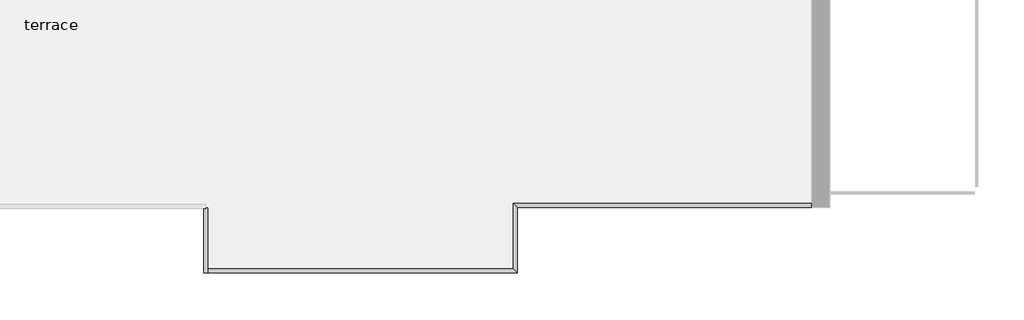
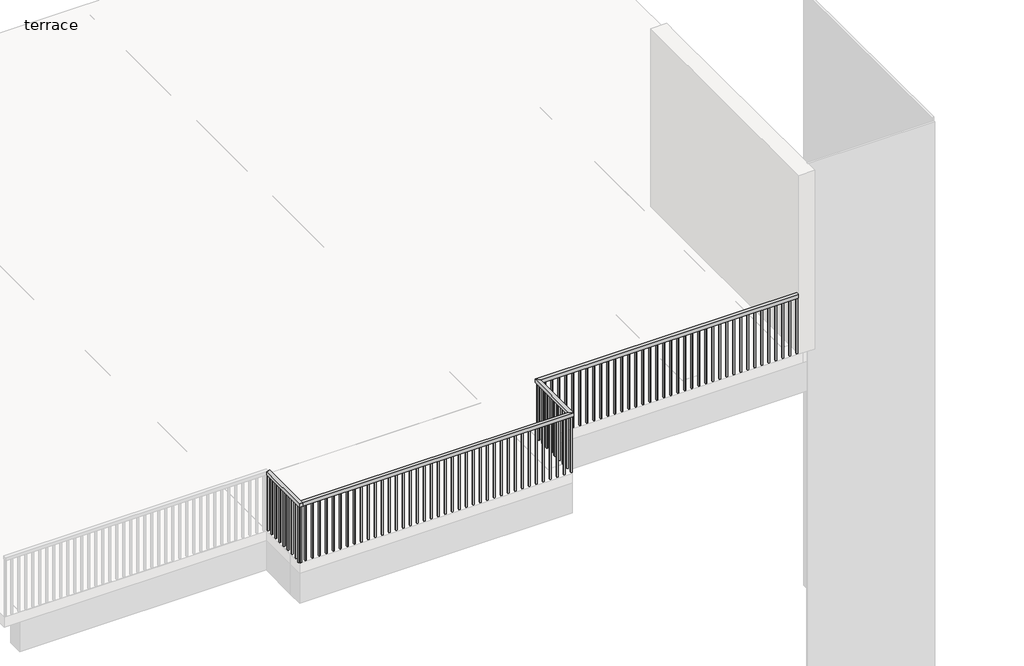
# One storey, part 3 of 6: 2 railings.
"""IFC4 building model written with IfcOpenShell, lengths in millimetres."""

from ifc_helpers import new_model, si_unit, frame, origin, place, context, project, spatial, polyline, outline, extrude, faceted_brep, element, save

model = new_model("IFC4")

# Units and contexts
model_context = context("Model", 3, world=origin())
ifc_project = project(units=[si_unit("LENGTHUNIT", "METRE", prefix="MILLI")], contexts=[model_context])

# Site, building, storey
site = spatial("IfcSite", under=ifc_project)
building = spatial("IfcBuilding", under=site)
storey = spatial("IfcBuildingStorey", under=building, Name="terrace", Elevation=7010.4)

# Railings
placement = place(None, origin())
element("IfcRailing", 1, ObjectType="Handrail - Rectangular", at=placement, inside=storey, context=model_context, shape_type="SweptSolid", body=[
    extrude(outline(polyline([(-12496.9493763, -4611.6564015), (-12446.1493763, -4611.6564015), (-12446.1493763, -5443.5064015), (-12496.9493763, -5443.5064015), (-12496.9493763, -4611.6564015)])), frame((0.0, 0.0, 7874.0), z_axis=(0.0, 0.0, 1.0), x_axis=(1.0, 0.0, 0.0)), (0.0, 0.0, 1.0), 50.8),
    extrude(outline(polyline([(-12481.0743763, -5414.9314015), (-12462.0243763, -5414.9314015), (-12462.0243763, -5433.9814015), (-12481.0743763, -5433.9814015), (-12481.0743763, -5414.9314015)])), frame((0.0, 0.0, 7010.4), z_axis=(0.0, 0.0, 1.0), x_axis=(1.0, 0.0, 0.0)), (0.0, 0.0, 1.0), 863.6),
    extrude(outline(polyline([(-12481.0743763, -5313.3314015), (-12462.0243763, -5313.3314015), (-12462.0243763, -5332.3814015), (-12481.0743763, -5332.3814015), (-12481.0743763, -5313.3314015)])), frame((0.0, 0.0, 7010.4), z_axis=(0.0, 0.0, 1.0), x_axis=(1.0, 0.0, 0.0)), (0.0, 0.0, 1.0), 863.6),
    extrude(outline(polyline([(-12481.0743763, -5211.7314015), (-12462.0243763, -5211.7314015), (-12462.0243763, -5230.7814015), (-12481.0743763, -5230.7814015), (-12481.0743763, -5211.7314015)])), frame((0.0, 0.0, 7010.4), z_axis=(0.0, 0.0, 1.0), x_axis=(1.0, 0.0, 0.0)), (0.0, 0.0, 1.0), 863.6),
    extrude(outline(polyline([(-12481.0743763, -5110.1314015), (-12462.0243763, -5110.1314015), (-12462.0243763, -5129.1814015), (-12481.0743763, -5129.1814015), (-12481.0743763, -5110.1314015)])), frame((0.0, 0.0, 7010.4), z_axis=(0.0, 0.0, 1.0), x_axis=(1.0, 0.0, 0.0)), (0.0, 0.0, 1.0), 863.6),
    extrude(outline(polyline([(-12481.0743763, -5008.5314015), (-12462.0243763, -5008.5314015), (-12462.0243763, -5027.5814015), (-12481.0743763, -5027.5814015), (-12481.0743763, -5008.5314015)])), frame((0.0, 0.0, 7010.4), z_axis=(0.0, 0.0, 1.0), x_axis=(1.0, 0.0, 0.0)), (0.0, 0.0, 1.0), 863.6),
    extrude(outline(polyline([(-12481.0743763, -4906.9314015), (-12462.0243763, -4906.9314015), (-12462.0243763, -4925.9814015), (-12481.0743763, -4925.9814015), (-12481.0743763, -4906.9314015)])), frame((0.0, 0.0, 7010.4), z_axis=(0.0, 0.0, 1.0), x_axis=(1.0, 0.0, 0.0)), (0.0, 0.0, 1.0), 863.6),
    extrude(outline(polyline([(-12481.0743763, -4805.3314015), (-12462.0243763, -4805.3314015), (-12462.0243763, -4824.3814015), (-12481.0743763, -4824.3814015), (-12481.0743763, -4805.3314015)])), frame((0.0, 0.0, 7010.4), z_axis=(0.0, 0.0, 1.0), x_axis=(1.0, 0.0, 0.0)), (0.0, 0.0, 1.0), 863.6),
    extrude(outline(polyline([(-12481.0743763, -4703.7314015), (-12462.0243763, -4703.7314015), (-12462.0243763, -4722.7814015), (-12481.0743763, -4722.7814015), (-12481.0743763, -4703.7314015)])), frame((0.0, 0.0, 7010.4), z_axis=(0.0, 0.0, 1.0), x_axis=(1.0, 0.0, 0.0)), (0.0, 0.0, 1.0), 863.6),
    extrude(outline(polyline([(-12481.0743763, -5424.4564015), (-12462.0243763, -5424.4564015), (-12462.0243763, -5443.5064015), (-12481.0743763, -5443.5064015), (-12481.0743763, -5424.4564015)])), frame((0.0, 0.0, 7010.4), z_axis=(0.0, 0.0, 1.0), x_axis=(1.0, 0.0, 0.0)), (0.0, 0.0, 1.0), 863.6),
    extrude(outline(polyline([(-12481.0743763, -4611.6564015), (-12462.0243763, -4611.6564015), (-12462.0243763, -4630.7064015), (-12481.0743763, -4630.7064015), (-12481.0743763, -4611.6564015)])), frame((0.0, 0.0, 7010.4), z_axis=(0.0, 0.0, 1.0), x_axis=(1.0, 0.0, 0.0)), (0.0, 0.0, 1.0), 863.6),
])
element("IfcRailing", 2, ObjectType="Handrail - Rectangular", at=placement, inside=storey, context=model_context, shape_type="SolidModel", body=[
    faceted_brep([(-12494.5077606, -5392.7064015, 7924.8), (-12494.5077606, -5392.7064015, 7874.0), (-12494.5077606, -5443.5064015, 7874.0), (-12494.5077606, -5443.5064015, 7924.8), (-8557.5077606, -5392.7064015, 7924.8), (-8557.5077606, -5392.7064015, 7874.0), (-8506.7077606, -5443.5064015, 7874.0), (-8506.7077606, -5443.5064015, 7924.8), (-8557.5077606, -4554.5064015, 7924.8), (-8557.5077606, -4554.5064015, 7874.0), (-8506.7077606, -4605.3064015, 7874.0), (-8506.7077606, -4605.3064015, 7924.8), (-4645.9077606, -4554.5064015, 7924.8), (-4645.9077606, -4605.3064015, 7924.8), (-4645.9077606, -4605.3064015, 7874.0), (-4645.9077606, -4554.5064015, 7874.0)], [[[0, 1, 2, 3]], [[1, 0, 4, 5]], [[2, 1, 5, 6]], [[3, 2, 6, 7]], [[0, 3, 7, 4]], [[5, 4, 8, 9]], [[6, 5, 9, 10]], [[7, 6, 10, 11]], [[4, 7, 11, 8]], [[12, 13, 14, 15]], [[9, 8, 12, 15]], [[10, 9, 15, 14]], [[11, 10, 14, 13]], [[8, 11, 13, 12]]]),
    extrude(outline(polyline([(-4680.8327606, -4589.4314015), (-4680.8327606, -4570.3814015), (-4661.7827606, -4570.3814015), (-4661.7827606, -4589.4314015), (-4680.8327606, -4589.4314015)])), frame((0.0, 0.0, 7010.4), z_axis=(0.0, 0.0, 1.0), x_axis=(1.0, 0.0, 0.0)), (0.0, 0.0, 1.0), 863.6),
    extrude(outline(polyline([(-4782.4327606, -4589.4314015), (-4782.4327606, -4570.3814015), (-4763.3827606, -4570.3814015), (-4763.3827606, -4589.4314015), (-4782.4327606, -4589.4314015)])), frame((0.0, 0.0, 7010.4), z_axis=(0.0, 0.0, 1.0), x_axis=(1.0, 0.0, 0.0)), (0.0, 0.0, 1.0), 863.6),
    extrude(outline(polyline([(-4884.0327606, -4589.4314015), (-4884.0327606, -4570.3814015), (-4864.9827606, -4570.3814015), (-4864.9827606, -4589.4314015), (-4884.0327606, -4589.4314015)])), frame((0.0, 0.0, 7010.4), z_axis=(0.0, 0.0, 1.0), x_axis=(1.0, 0.0, 0.0)), (0.0, 0.0, 1.0), 863.6),
    extrude(outline(polyline([(-4985.6327606, -4589.4314015), (-4985.6327606, -4570.3814015), (-4966.5827606, -4570.3814015), (-4966.5827606, -4589.4314015), (-4985.6327606, -4589.4314015)])), frame((0.0, 0.0, 7010.4), z_axis=(0.0, 0.0, 1.0), x_axis=(1.0, 0.0, 0.0)), (0.0, 0.0, 1.0), 863.6),
    extrude(outline(polyline([(-5087.2327606, -4589.4314015), (-5087.2327606, -4570.3814015), (-5068.1827606, -4570.3814015), (-5068.1827606, -4589.4314015), (-5087.2327606, -4589.4314015)])), frame((0.0, 0.0, 7010.4), z_axis=(0.0, 0.0, 1.0), x_axis=(1.0, 0.0, 0.0)), (0.0, 0.0, 1.0), 863.6),
    extrude(outline(polyline([(-5188.8327606, -4589.4314015), (-5188.8327606, -4570.3814015), (-5169.7827606, -4570.3814015), (-5169.7827606, -4589.4314015), (-5188.8327606, -4589.4314015)])), frame((0.0, 0.0, 7010.4), z_axis=(0.0, 0.0, 1.0), x_axis=(1.0, 0.0, 0.0)), (0.0, 0.0, 1.0), 863.6),
    extrude(outline(polyline([(-5290.4327606, -4589.4314015), (-5290.4327606, -4570.3814015), (-5271.3827606, -4570.3814015), (-5271.3827606, -4589.4314015), (-5290.4327606, -4589.4314015)])), frame((0.0, 0.0, 7010.4), z_axis=(0.0, 0.0, 1.0), x_axis=(1.0, 0.0, 0.0)), (0.0, 0.0, 1.0), 863.6),
    extrude(outline(polyline([(-5392.0327606, -4589.4314015), (-5392.0327606, -4570.3814015), (-5372.9827606, -4570.3814015), (-5372.9827606, -4589.4314015), (-5392.0327606, -4589.4314015)])), frame((0.0, 0.0, 7010.4), z_axis=(0.0, 0.0, 1.0), x_axis=(1.0, 0.0, 0.0)), (0.0, 0.0, 1.0), 863.6),
    extrude(outline(polyline([(-5493.6327606, -4589.4314015), (-5493.6327606, -4570.3814015), (-5474.5827606, -4570.3814015), (-5474.5827606, -4589.4314015), (-5493.6327606, -4589.4314015)])), frame((0.0, 0.0, 7010.4), z_axis=(0.0, 0.0, 1.0), x_axis=(1.0, 0.0, 0.0)), (0.0, 0.0, 1.0), 863.6),
    extrude(outline(polyline([(-5595.2327606, -4589.4314015), (-5595.2327606, -4570.3814015), (-5576.1827606, -4570.3814015), (-5576.1827606, -4589.4314015), (-5595.2327606, -4589.4314015)])), frame((0.0, 0.0, 7010.4), z_axis=(0.0, 0.0, 1.0), x_axis=(1.0, 0.0, 0.0)), (0.0, 0.0, 1.0), 863.6),
    extrude(outline(polyline([(-5696.8327606, -4589.4314015), (-5696.8327606, -4570.3814015), (-5677.7827606, -4570.3814015), (-5677.7827606, -4589.4314015), (-5696.8327606, -4589.4314015)])), frame((0.0, 0.0, 7010.4), z_axis=(0.0, 0.0, 1.0), x_axis=(1.0, 0.0, 0.0)), (0.0, 0.0, 1.0), 863.6),
    extrude(outline(polyline([(-5798.4327606, -4589.4314015), (-5798.4327606, -4570.3814015), (-5779.3827606, -4570.3814015), (-5779.3827606, -4589.4314015), (-5798.4327606, -4589.4314015)])), frame((0.0, 0.0, 7010.4), z_axis=(0.0, 0.0, 1.0), x_axis=(1.0, 0.0, 0.0)), (0.0, 0.0, 1.0), 863.6),
    extrude(outline(polyline([(-5900.0327606, -4589.4314015), (-5900.0327606, -4570.3814015), (-5880.9827606, -4570.3814015), (-5880.9827606, -4589.4314015), (-5900.0327606, -4589.4314015)])), frame((0.0, 0.0, 7010.4), z_axis=(0.0, 0.0, 1.0), x_axis=(1.0, 0.0, 0.0)), (0.0, 0.0, 1.0), 863.6),
    extrude(outline(polyline([(-6001.6327606, -4589.4314015), (-6001.6327606, -4570.3814015), (-5982.5827606, -4570.3814015), (-5982.5827606, -4589.4314015), (-6001.6327606, -4589.4314015)])), frame((0.0, 0.0, 7010.4), z_axis=(0.0, 0.0, 1.0), x_axis=(1.0, 0.0, 0.0)), (0.0, 0.0, 1.0), 863.6),
    extrude(outline(polyline([(-6103.2327606, -4589.4314015), (-6103.2327606, -4570.3814015), (-6084.1827606, -4570.3814015), (-6084.1827606, -4589.4314015), (-6103.2327606, -4589.4314015)])), frame((0.0, 0.0, 7010.4), z_axis=(0.0, 0.0, 1.0), x_axis=(1.0, 0.0, 0.0)), (0.0, 0.0, 1.0), 863.6),
    extrude(outline(polyline([(-6204.8327606, -4589.4314015), (-6204.8327606, -4570.3814015), (-6185.7827606, -4570.3814015), (-6185.7827606, -4589.4314015), (-6204.8327606, -4589.4314015)])), frame((0.0, 0.0, 7010.4), z_axis=(0.0, 0.0, 1.0), x_axis=(1.0, 0.0, 0.0)), (0.0, 0.0, 1.0), 863.6),
    extrude(outline(polyline([(-6306.4327606, -4589.4314015), (-6306.4327606, -4570.3814015), (-6287.3827606, -4570.3814015), (-6287.3827606, -4589.4314015), (-6306.4327606, -4589.4314015)])), frame((0.0, 0.0, 7010.4), z_axis=(0.0, 0.0, 1.0), x_axis=(1.0, 0.0, 0.0)), (0.0, 0.0, 1.0), 863.6),
    extrude(outline(polyline([(-6408.0327606, -4589.4314015), (-6408.0327606, -4570.3814015), (-6388.9827606, -4570.3814015), (-6388.9827606, -4589.4314015), (-6408.0327606, -4589.4314015)])), frame((0.0, 0.0, 7010.4), z_axis=(0.0, 0.0, 1.0), x_axis=(1.0, 0.0, 0.0)), (0.0, 0.0, 1.0), 863.6),
    extrude(outline(polyline([(-6509.6327606, -4589.4314015), (-6509.6327606, -4570.3814015), (-6490.5827606, -4570.3814015), (-6490.5827606, -4589.4314015), (-6509.6327606, -4589.4314015)])), frame((0.0, 0.0, 7010.4), z_axis=(0.0, 0.0, 1.0), x_axis=(1.0, 0.0, 0.0)), (0.0, 0.0, 1.0), 863.6),
    extrude(outline(polyline([(-6611.2327606, -4589.4314015), (-6611.2327606, -4570.3814015), (-6592.1827606, -4570.3814015), (-6592.1827606, -4589.4314015), (-6611.2327606, -4589.4314015)])), frame((0.0, 0.0, 7010.4), z_axis=(0.0, 0.0, 1.0), x_axis=(1.0, 0.0, 0.0)), (0.0, 0.0, 1.0), 863.6),
    extrude(outline(polyline([(-6712.8327606, -4589.4314015), (-6712.8327606, -4570.3814015), (-6693.7827606, -4570.3814015), (-6693.7827606, -4589.4314015), (-6712.8327606, -4589.4314015)])), frame((0.0, 0.0, 7010.4), z_axis=(0.0, 0.0, 1.0), x_axis=(1.0, 0.0, 0.0)), (0.0, 0.0, 1.0), 863.6),
    extrude(outline(polyline([(-6814.4327606, -4589.4314015), (-6814.4327606, -4570.3814015), (-6795.3827606, -4570.3814015), (-6795.3827606, -4589.4314015), (-6814.4327606, -4589.4314015)])), frame((0.0, 0.0, 7010.4), z_axis=(0.0, 0.0, 1.0), x_axis=(1.0, 0.0, 0.0)), (0.0, 0.0, 1.0), 863.6),
    extrude(outline(polyline([(-6916.0327606, -4589.4314015), (-6916.0327606, -4570.3814015), (-6896.9827606, -4570.3814015), (-6896.9827606, -4589.4314015), (-6916.0327606, -4589.4314015)])), frame((0.0, 0.0, 7010.4), z_axis=(0.0, 0.0, 1.0), x_axis=(1.0, 0.0, 0.0)), (0.0, 0.0, 1.0), 863.6),
    extrude(outline(polyline([(-7017.6327606, -4589.4314015), (-7017.6327606, -4570.3814015), (-6998.5827606, -4570.3814015), (-6998.5827606, -4589.4314015), (-7017.6327606, -4589.4314015)])), frame((0.0, 0.0, 7010.4), z_axis=(0.0, 0.0, 1.0), x_axis=(1.0, 0.0, 0.0)), (0.0, 0.0, 1.0), 863.6),
    extrude(outline(polyline([(-7119.2327606, -4589.4314015), (-7119.2327606, -4570.3814015), (-7100.1827606, -4570.3814015), (-7100.1827606, -4589.4314015), (-7119.2327606, -4589.4314015)])), frame((0.0, 0.0, 7010.4), z_axis=(0.0, 0.0, 1.0), x_axis=(1.0, 0.0, 0.0)), (0.0, 0.0, 1.0), 863.6),
    extrude(outline(polyline([(-7220.8327606, -4589.4314015), (-7220.8327606, -4570.3814015), (-7201.7827606, -4570.3814015), (-7201.7827606, -4589.4314015), (-7220.8327606, -4589.4314015)])), frame((0.0, 0.0, 7010.4), z_axis=(0.0, 0.0, 1.0), x_axis=(1.0, 0.0, 0.0)), (0.0, 0.0, 1.0), 863.6),
    extrude(outline(polyline([(-7322.4327606, -4589.4314015), (-7322.4327606, -4570.3814015), (-7303.3827606, -4570.3814015), (-7303.3827606, -4589.4314015), (-7322.4327606, -4589.4314015)])), frame((0.0, 0.0, 7010.4), z_axis=(0.0, 0.0, 1.0), x_axis=(1.0, 0.0, 0.0)), (0.0, 0.0, 1.0), 863.6),
    extrude(outline(polyline([(-7424.0327606, -4589.4314015), (-7424.0327606, -4570.3814015), (-7404.9827606, -4570.3814015), (-7404.9827606, -4589.4314015), (-7424.0327606, -4589.4314015)])), frame((0.0, 0.0, 7010.4), z_axis=(0.0, 0.0, 1.0), x_axis=(1.0, 0.0, 0.0)), (0.0, 0.0, 1.0), 863.6),
    extrude(outline(polyline([(-7525.6327606, -4589.4314015), (-7525.6327606, -4570.3814015), (-7506.5827606, -4570.3814015), (-7506.5827606, -4589.4314015), (-7525.6327606, -4589.4314015)])), frame((0.0, 0.0, 7010.4), z_axis=(0.0, 0.0, 1.0), x_axis=(1.0, 0.0, 0.0)), (0.0, 0.0, 1.0), 863.6),
    extrude(outline(polyline([(-7627.2327606, -4589.4314015), (-7627.2327606, -4570.3814015), (-7608.1827606, -4570.3814015), (-7608.1827606, -4589.4314015), (-7627.2327606, -4589.4314015)])), frame((0.0, 0.0, 7010.4), z_axis=(0.0, 0.0, 1.0), x_axis=(1.0, 0.0, 0.0)), (0.0, 0.0, 1.0), 863.6),
    extrude(outline(polyline([(-7728.8327606, -4589.4314015), (-7728.8327606, -4570.3814015), (-7709.7827606, -4570.3814015), (-7709.7827606, -4589.4314015), (-7728.8327606, -4589.4314015)])), frame((0.0, 0.0, 7010.4), z_axis=(0.0, 0.0, 1.0), x_axis=(1.0, 0.0, 0.0)), (0.0, 0.0, 1.0), 863.6),
    extrude(outline(polyline([(-7830.4327606, -4589.4314015), (-7830.4327606, -4570.3814015), (-7811.3827606, -4570.3814015), (-7811.3827606, -4589.4314015), (-7830.4327606, -4589.4314015)])), frame((0.0, 0.0, 7010.4), z_axis=(0.0, 0.0, 1.0), x_axis=(1.0, 0.0, 0.0)), (0.0, 0.0, 1.0), 863.6),
    extrude(outline(polyline([(-7932.0327606, -4589.4314015), (-7932.0327606, -4570.3814015), (-7912.9827606, -4570.3814015), (-7912.9827606, -4589.4314015), (-7932.0327606, -4589.4314015)])), frame((0.0, 0.0, 7010.4), z_axis=(0.0, 0.0, 1.0), x_axis=(1.0, 0.0, 0.0)), (0.0, 0.0, 1.0), 863.6),
    extrude(outline(polyline([(-8033.6327606, -4589.4314015), (-8033.6327606, -4570.3814015), (-8014.5827606, -4570.3814015), (-8014.5827606, -4589.4314015), (-8033.6327606, -4589.4314015)])), frame((0.0, 0.0, 7010.4), z_axis=(0.0, 0.0, 1.0), x_axis=(1.0, 0.0, 0.0)), (0.0, 0.0, 1.0), 863.6),
    extrude(outline(polyline([(-8135.2327606, -4589.4314015), (-8135.2327606, -4570.3814015), (-8116.1827606, -4570.3814015), (-8116.1827606, -4589.4314015), (-8135.2327606, -4589.4314015)])), frame((0.0, 0.0, 7010.4), z_axis=(0.0, 0.0, 1.0), x_axis=(1.0, 0.0, 0.0)), (0.0, 0.0, 1.0), 863.6),
    extrude(outline(polyline([(-8236.8327606, -4589.4314015), (-8236.8327606, -4570.3814015), (-8217.7827606, -4570.3814015), (-8217.7827606, -4589.4314015), (-8236.8327606, -4589.4314015)])), frame((0.0, 0.0, 7010.4), z_axis=(0.0, 0.0, 1.0), x_axis=(1.0, 0.0, 0.0)), (0.0, 0.0, 1.0), 863.6),
    extrude(outline(polyline([(-8338.4327606, -4589.4314015), (-8338.4327606, -4570.3814015), (-8319.3827606, -4570.3814015), (-8319.3827606, -4589.4314015), (-8338.4327606, -4589.4314015)])), frame((0.0, 0.0, 7010.4), z_axis=(0.0, 0.0, 1.0), x_axis=(1.0, 0.0, 0.0)), (0.0, 0.0, 1.0), 863.6),
    extrude(outline(polyline([(-8440.0327606, -4589.4314015), (-8440.0327606, -4570.3814015), (-8420.9827606, -4570.3814015), (-8420.9827606, -4589.4314015), (-8440.0327606, -4589.4314015)])), frame((0.0, 0.0, 7010.4), z_axis=(0.0, 0.0, 1.0), x_axis=(1.0, 0.0, 0.0)), (0.0, 0.0, 1.0), 863.6),
    extrude(outline(polyline([(-8522.5827606, -4614.8314015), (-8541.6327606, -4614.8314015), (-8541.6327606, -4595.7814015), (-8522.5827606, -4595.7814015), (-8522.5827606, -4614.8314015)])), frame((0.0, 0.0, 7010.4), z_axis=(0.0, 0.0, 1.0), x_axis=(1.0, 0.0, 0.0)), (0.0, 0.0, 1.0), 863.6),
    extrude(outline(polyline([(-8522.5827606, -4716.4314015), (-8541.6327606, -4716.4314015), (-8541.6327606, -4697.3814015), (-8522.5827606, -4697.3814015), (-8522.5827606, -4716.4314015)])), frame((0.0, 0.0, 7010.4), z_axis=(0.0, 0.0, 1.0), x_axis=(1.0, 0.0, 0.0)), (0.0, 0.0, 1.0), 863.6),
    extrude(outline(polyline([(-8522.5827606, -4818.0314015), (-8541.6327606, -4818.0314015), (-8541.6327606, -4798.9814015), (-8522.5827606, -4798.9814015), (-8522.5827606, -4818.0314015)])), frame((0.0, 0.0, 7010.4), z_axis=(0.0, 0.0, 1.0), x_axis=(1.0, 0.0, 0.0)), (0.0, 0.0, 1.0), 863.6),
    extrude(outline(polyline([(-8522.5827606, -4919.6314015), (-8541.6327606, -4919.6314015), (-8541.6327606, -4900.5814015), (-8522.5827606, -4900.5814015), (-8522.5827606, -4919.6314015)])), frame((0.0, 0.0, 7010.4), z_axis=(0.0, 0.0, 1.0), x_axis=(1.0, 0.0, 0.0)), (0.0, 0.0, 1.0), 863.6),
    extrude(outline(polyline([(-8522.5827606, -5021.2314015), (-8541.6327606, -5021.2314015), (-8541.6327606, -5002.1814015), (-8522.5827606, -5002.1814015), (-8522.5827606, -5021.2314015)])), frame((0.0, 0.0, 7010.4), z_axis=(0.0, 0.0, 1.0), x_axis=(1.0, 0.0, 0.0)), (0.0, 0.0, 1.0), 863.6),
    extrude(outline(polyline([(-8522.5827606, -5122.8314015), (-8541.6327606, -5122.8314015), (-8541.6327606, -5103.7814015), (-8522.5827606, -5103.7814015), (-8522.5827606, -5122.8314015)])), frame((0.0, 0.0, 7010.4), z_axis=(0.0, 0.0, 1.0), x_axis=(1.0, 0.0, 0.0)), (0.0, 0.0, 1.0), 863.6),
    extrude(outline(polyline([(-8522.5827606, -5224.4314015), (-8541.6327606, -5224.4314015), (-8541.6327606, -5205.3814015), (-8522.5827606, -5205.3814015), (-8522.5827606, -5224.4314015)])), frame((0.0, 0.0, 7010.4), z_axis=(0.0, 0.0, 1.0), x_axis=(1.0, 0.0, 0.0)), (0.0, 0.0, 1.0), 863.6),
    extrude(outline(polyline([(-8522.5827606, -5326.0314015), (-8541.6327606, -5326.0314015), (-8541.6327606, -5306.9814015), (-8522.5827606, -5306.9814015), (-8522.5827606, -5326.0314015)])), frame((0.0, 0.0, 7010.4), z_axis=(0.0, 0.0, 1.0), x_axis=(1.0, 0.0, 0.0)), (0.0, 0.0, 1.0), 863.6),
    extrude(outline(polyline([(-8643.2327606, -5427.6314015), (-8643.2327606, -5408.5814015), (-8624.1827606, -5408.5814015), (-8624.1827606, -5427.6314015), (-8643.2327606, -5427.6314015)])), frame((0.0, 0.0, 7010.4), z_axis=(0.0, 0.0, 1.0), x_axis=(1.0, 0.0, 0.0)), (0.0, 0.0, 1.0), 863.6),
    extrude(outline(polyline([(-8744.8327606, -5427.6314015), (-8744.8327606, -5408.5814015), (-8725.7827606, -5408.5814015), (-8725.7827606, -5427.6314015), (-8744.8327606, -5427.6314015)])), frame((0.0, 0.0, 7010.4), z_axis=(0.0, 0.0, 1.0), x_axis=(1.0, 0.0, 0.0)), (0.0, 0.0, 1.0), 863.6),
    extrude(outline(polyline([(-8846.4327606, -5427.6314015), (-8846.4327606, -5408.5814015), (-8827.3827606, -5408.5814015), (-8827.3827606, -5427.6314015), (-8846.4327606, -5427.6314015)])), frame((0.0, 0.0, 7010.4), z_axis=(0.0, 0.0, 1.0), x_axis=(1.0, 0.0, 0.0)), (0.0, 0.0, 1.0), 863.6),
    extrude(outline(polyline([(-8948.0327606, -5427.6314015), (-8948.0327606, -5408.5814015), (-8928.9827606, -5408.5814015), (-8928.9827606, -5427.6314015), (-8948.0327606, -5427.6314015)])), frame((0.0, 0.0, 7010.4), z_axis=(0.0, 0.0, 1.0), x_axis=(1.0, 0.0, 0.0)), (0.0, 0.0, 1.0), 863.6),
    extrude(outline(polyline([(-9049.6327606, -5427.6314015), (-9049.6327606, -5408.5814015), (-9030.5827606, -5408.5814015), (-9030.5827606, -5427.6314015), (-9049.6327606, -5427.6314015)])), frame((0.0, 0.0, 7010.4), z_axis=(0.0, 0.0, 1.0), x_axis=(1.0, 0.0, 0.0)), (0.0, 0.0, 1.0), 863.6),
    extrude(outline(polyline([(-9151.2327606, -5427.6314015), (-9151.2327606, -5408.5814015), (-9132.1827606, -5408.5814015), (-9132.1827606, -5427.6314015), (-9151.2327606, -5427.6314015)])), frame((0.0, 0.0, 7010.4), z_axis=(0.0, 0.0, 1.0), x_axis=(1.0, 0.0, 0.0)), (0.0, 0.0, 1.0), 863.6),
    extrude(outline(polyline([(-9252.8327606, -5427.6314015), (-9252.8327606, -5408.5814015), (-9233.7827606, -5408.5814015), (-9233.7827606, -5427.6314015), (-9252.8327606, -5427.6314015)])), frame((0.0, 0.0, 7010.4), z_axis=(0.0, 0.0, 1.0), x_axis=(1.0, 0.0, 0.0)), (0.0, 0.0, 1.0), 863.6),
    extrude(outline(polyline([(-9354.4327606, -5427.6314015), (-9354.4327606, -5408.5814015), (-9335.3827606, -5408.5814015), (-9335.3827606, -5427.6314015), (-9354.4327606, -5427.6314015)])), frame((0.0, 0.0, 7010.4), z_axis=(0.0, 0.0, 1.0), x_axis=(1.0, 0.0, 0.0)), (0.0, 0.0, 1.0), 863.6),
    extrude(outline(polyline([(-9456.0327606, -5427.6314015), (-9456.0327606, -5408.5814015), (-9436.9827606, -5408.5814015), (-9436.9827606, -5427.6314015), (-9456.0327606, -5427.6314015)])), frame((0.0, 0.0, 7010.4), z_axis=(0.0, 0.0, 1.0), x_axis=(1.0, 0.0, 0.0)), (0.0, 0.0, 1.0), 863.6),
    extrude(outline(polyline([(-9557.6327606, -5427.6314015), (-9557.6327606, -5408.5814015), (-9538.5827606, -5408.5814015), (-9538.5827606, -5427.6314015), (-9557.6327606, -5427.6314015)])), frame((0.0, 0.0, 7010.4), z_axis=(0.0, 0.0, 1.0), x_axis=(1.0, 0.0, 0.0)), (0.0, 0.0, 1.0), 863.6),
    extrude(outline(polyline([(-9659.2327606, -5427.6314015), (-9659.2327606, -5408.5814015), (-9640.1827606, -5408.5814015), (-9640.1827606, -5427.6314015), (-9659.2327606, -5427.6314015)])), frame((0.0, 0.0, 7010.4), z_axis=(0.0, 0.0, 1.0), x_axis=(1.0, 0.0, 0.0)), (0.0, 0.0, 1.0), 863.6),
    extrude(outline(polyline([(-9760.8327606, -5427.6314015), (-9760.8327606, -5408.5814015), (-9741.7827606, -5408.5814015), (-9741.7827606, -5427.6314015), (-9760.8327606, -5427.6314015)])), frame((0.0, 0.0, 7010.4), z_axis=(0.0, 0.0, 1.0), x_axis=(1.0, 0.0, 0.0)), (0.0, 0.0, 1.0), 863.6),
    extrude(outline(polyline([(-9862.4327606, -5427.6314015), (-9862.4327606, -5408.5814015), (-9843.3827606, -5408.5814015), (-9843.3827606, -5427.6314015), (-9862.4327606, -5427.6314015)])), frame((0.0, 0.0, 7010.4), z_axis=(0.0, 0.0, 1.0), x_axis=(1.0, 0.0, 0.0)), (0.0, 0.0, 1.0), 863.6),
    extrude(outline(polyline([(-9964.0327606, -5427.6314015), (-9964.0327606, -5408.5814015), (-9944.9827606, -5408.5814015), (-9944.9827606, -5427.6314015), (-9964.0327606, -5427.6314015)])), frame((0.0, 0.0, 7010.4), z_axis=(0.0, 0.0, 1.0), x_axis=(1.0, 0.0, 0.0)), (0.0, 0.0, 1.0), 863.6),
    extrude(outline(polyline([(-10065.6327606, -5427.6314015), (-10065.6327606, -5408.5814015), (-10046.5827606, -5408.5814015), (-10046.5827606, -5427.6314015), (-10065.6327606, -5427.6314015)])), frame((0.0, 0.0, 7010.4), z_axis=(0.0, 0.0, 1.0), x_axis=(1.0, 0.0, 0.0)), (0.0, 0.0, 1.0), 863.6),
    extrude(outline(polyline([(-10167.2327606, -5427.6314015), (-10167.2327606, -5408.5814015), (-10148.1827606, -5408.5814015), (-10148.1827606, -5427.6314015), (-10167.2327606, -5427.6314015)])), frame((0.0, 0.0, 7010.4), z_axis=(0.0, 0.0, 1.0), x_axis=(1.0, 0.0, 0.0)), (0.0, 0.0, 1.0), 863.6),
    extrude(outline(polyline([(-10268.8327606, -5427.6314015), (-10268.8327606, -5408.5814015), (-10249.7827606, -5408.5814015), (-10249.7827606, -5427.6314015), (-10268.8327606, -5427.6314015)])), frame((0.0, 0.0, 7010.4), z_axis=(0.0, 0.0, 1.0), x_axis=(1.0, 0.0, 0.0)), (0.0, 0.0, 1.0), 863.6),
    extrude(outline(polyline([(-10370.4327606, -5427.6314015), (-10370.4327606, -5408.5814015), (-10351.3827606, -5408.5814015), (-10351.3827606, -5427.6314015), (-10370.4327606, -5427.6314015)])), frame((0.0, 0.0, 7010.4), z_axis=(0.0, 0.0, 1.0), x_axis=(1.0, 0.0, 0.0)), (0.0, 0.0, 1.0), 863.6),
    extrude(outline(polyline([(-10472.0327606, -5427.6314015), (-10472.0327606, -5408.5814015), (-10452.9827606, -5408.5814015), (-10452.9827606, -5427.6314015), (-10472.0327606, -5427.6314015)])), frame((0.0, 0.0, 7010.4), z_axis=(0.0, 0.0, 1.0), x_axis=(1.0, 0.0, 0.0)), (0.0, 0.0, 1.0), 863.6),
    extrude(outline(polyline([(-10573.6327606, -5427.6314015), (-10573.6327606, -5408.5814015), (-10554.5827606, -5408.5814015), (-10554.5827606, -5427.6314015), (-10573.6327606, -5427.6314015)])), frame((0.0, 0.0, 7010.4), z_axis=(0.0, 0.0, 1.0), x_axis=(1.0, 0.0, 0.0)), (0.0, 0.0, 1.0), 863.6),
    extrude(outline(polyline([(-10675.2327606, -5427.6314015), (-10675.2327606, -5408.5814015), (-10656.1827606, -5408.5814015), (-10656.1827606, -5427.6314015), (-10675.2327606, -5427.6314015)])), frame((0.0, 0.0, 7010.4), z_axis=(0.0, 0.0, 1.0), x_axis=(1.0, 0.0, 0.0)), (0.0, 0.0, 1.0), 863.6),
    extrude(outline(polyline([(-10776.8327606, -5427.6314015), (-10776.8327606, -5408.5814015), (-10757.7827606, -5408.5814015), (-10757.7827606, -5427.6314015), (-10776.8327606, -5427.6314015)])), frame((0.0, 0.0, 7010.4), z_axis=(0.0, 0.0, 1.0), x_axis=(1.0, 0.0, 0.0)), (0.0, 0.0, 1.0), 863.6),
    extrude(outline(polyline([(-10878.4327606, -5427.6314015), (-10878.4327606, -5408.5814015), (-10859.3827606, -5408.5814015), (-10859.3827606, -5427.6314015), (-10878.4327606, -5427.6314015)])), frame((0.0, 0.0, 7010.4), z_axis=(0.0, 0.0, 1.0), x_axis=(1.0, 0.0, 0.0)), (0.0, 0.0, 1.0), 863.6),
    extrude(outline(polyline([(-10980.0327606, -5427.6314015), (-10980.0327606, -5408.5814015), (-10960.9827606, -5408.5814015), (-10960.9827606, -5427.6314015), (-10980.0327606, -5427.6314015)])), frame((0.0, 0.0, 7010.4), z_axis=(0.0, 0.0, 1.0), x_axis=(1.0, 0.0, 0.0)), (0.0, 0.0, 1.0), 863.6),
    extrude(outline(polyline([(-11081.6327606, -5427.6314015), (-11081.6327606, -5408.5814015), (-11062.5827606, -5408.5814015), (-11062.5827606, -5427.6314015), (-11081.6327606, -5427.6314015)])), frame((0.0, 0.0, 7010.4), z_axis=(0.0, 0.0, 1.0), x_axis=(1.0, 0.0, 0.0)), (0.0, 0.0, 1.0), 863.6),
    extrude(outline(polyline([(-11183.2327606, -5427.6314015), (-11183.2327606, -5408.5814015), (-11164.1827606, -5408.5814015), (-11164.1827606, -5427.6314015), (-11183.2327606, -5427.6314015)])), frame((0.0, 0.0, 7010.4), z_axis=(0.0, 0.0, 1.0), x_axis=(1.0, 0.0, 0.0)), (0.0, 0.0, 1.0), 863.6),
    extrude(outline(polyline([(-11284.8327606, -5427.6314015), (-11284.8327606, -5408.5814015), (-11265.7827606, -5408.5814015), (-11265.7827606, -5427.6314015), (-11284.8327606, -5427.6314015)])), frame((0.0, 0.0, 7010.4), z_axis=(0.0, 0.0, 1.0), x_axis=(1.0, 0.0, 0.0)), (0.0, 0.0, 1.0), 863.6),
    extrude(outline(polyline([(-11386.4327606, -5427.6314015), (-11386.4327606, -5408.5814015), (-11367.3827606, -5408.5814015), (-11367.3827606, -5427.6314015), (-11386.4327606, -5427.6314015)])), frame((0.0, 0.0, 7010.4), z_axis=(0.0, 0.0, 1.0), x_axis=(1.0, 0.0, 0.0)), (0.0, 0.0, 1.0), 863.6),
    extrude(outline(polyline([(-11488.0327606, -5427.6314015), (-11488.0327606, -5408.5814015), (-11468.9827606, -5408.5814015), (-11468.9827606, -5427.6314015), (-11488.0327606, -5427.6314015)])), frame((0.0, 0.0, 7010.4), z_axis=(0.0, 0.0, 1.0), x_axis=(1.0, 0.0, 0.0)), (0.0, 0.0, 1.0), 863.6),
    extrude(outline(polyline([(-11589.6327606, -5427.6314015), (-11589.6327606, -5408.5814015), (-11570.5827606, -5408.5814015), (-11570.5827606, -5427.6314015), (-11589.6327606, -5427.6314015)])), frame((0.0, 0.0, 7010.4), z_axis=(0.0, 0.0, 1.0), x_axis=(1.0, 0.0, 0.0)), (0.0, 0.0, 1.0), 863.6),
    extrude(outline(polyline([(-11691.2327606, -5427.6314015), (-11691.2327606, -5408.5814015), (-11672.1827606, -5408.5814015), (-11672.1827606, -5427.6314015), (-11691.2327606, -5427.6314015)])), frame((0.0, 0.0, 7010.4), z_axis=(0.0, 0.0, 1.0), x_axis=(1.0, 0.0, 0.0)), (0.0, 0.0, 1.0), 863.6),
    extrude(outline(polyline([(-11792.8327606, -5427.6314015), (-11792.8327606, -5408.5814015), (-11773.7827606, -5408.5814015), (-11773.7827606, -5427.6314015), (-11792.8327606, -5427.6314015)])), frame((0.0, 0.0, 7010.4), z_axis=(0.0, 0.0, 1.0), x_axis=(1.0, 0.0, 0.0)), (0.0, 0.0, 1.0), 863.6),
    extrude(outline(polyline([(-11894.4327606, -5427.6314015), (-11894.4327606, -5408.5814015), (-11875.3827606, -5408.5814015), (-11875.3827606, -5427.6314015), (-11894.4327606, -5427.6314015)])), frame((0.0, 0.0, 7010.4), z_axis=(0.0, 0.0, 1.0), x_axis=(1.0, 0.0, 0.0)), (0.0, 0.0, 1.0), 863.6),
    extrude(outline(polyline([(-11996.0327606, -5427.6314015), (-11996.0327606, -5408.5814015), (-11976.9827606, -5408.5814015), (-11976.9827606, -5427.6314015), (-11996.0327606, -5427.6314015)])), frame((0.0, 0.0, 7010.4), z_axis=(0.0, 0.0, 1.0), x_axis=(1.0, 0.0, 0.0)), (0.0, 0.0, 1.0), 863.6),
    extrude(outline(polyline([(-12097.6327606, -5427.6314015), (-12097.6327606, -5408.5814015), (-12078.5827606, -5408.5814015), (-12078.5827606, -5427.6314015), (-12097.6327606, -5427.6314015)])), frame((0.0, 0.0, 7010.4), z_axis=(0.0, 0.0, 1.0), x_axis=(1.0, 0.0, 0.0)), (0.0, 0.0, 1.0), 863.6),
    extrude(outline(polyline([(-12199.2327606, -5427.6314015), (-12199.2327606, -5408.5814015), (-12180.1827606, -5408.5814015), (-12180.1827606, -5427.6314015), (-12199.2327606, -5427.6314015)])), frame((0.0, 0.0, 7010.4), z_axis=(0.0, 0.0, 1.0), x_axis=(1.0, 0.0, 0.0)), (0.0, 0.0, 1.0), 863.6),
    extrude(outline(polyline([(-12300.8327606, -5427.6314015), (-12300.8327606, -5408.5814015), (-12281.7827606, -5408.5814015), (-12281.7827606, -5427.6314015), (-12300.8327606, -5427.6314015)])), frame((0.0, 0.0, 7010.4), z_axis=(0.0, 0.0, 1.0), x_axis=(1.0, 0.0, 0.0)), (0.0, 0.0, 1.0), 863.6),
    extrude(outline(polyline([(-12402.4327606, -5427.6314015), (-12402.4327606, -5408.5814015), (-12383.3827606, -5408.5814015), (-12383.3827606, -5427.6314015), (-12402.4327606, -5427.6314015)])), frame((0.0, 0.0, 7010.4), z_axis=(0.0, 0.0, 1.0), x_axis=(1.0, 0.0, 0.0)), (0.0, 0.0, 1.0), 863.6),
    extrude(outline(polyline([(-8522.5827606, -4589.4314015), (-8541.6327606, -4589.4314015), (-8541.6327606, -4570.3814015), (-8522.5827606, -4570.3814015), (-8522.5827606, -4589.4314015)])), frame((0.0, 0.0, 7010.4), z_axis=(0.0, 0.0, 1.0), x_axis=(1.0, 0.0, 0.0)), (0.0, 0.0, 1.0), 863.6),
    extrude(outline(polyline([(-8541.6327606, -5427.6314015), (-8541.6327606, -5408.5814015), (-8522.5827606, -5408.5814015), (-8522.5827606, -5427.6314015), (-8541.6327606, -5427.6314015)])), frame((0.0, 0.0, 7010.4), z_axis=(0.0, 0.0, 1.0), x_axis=(1.0, 0.0, 0.0)), (0.0, 0.0, 1.0), 863.6),
    extrude(outline(polyline([(-4664.9577606, -4589.4314015), (-4664.9577606, -4570.3814015), (-4645.9077606, -4570.3814015), (-4645.9077606, -4589.4314015), (-4664.9577606, -4589.4314015)])), frame((0.0, 0.0, 7010.4), z_axis=(0.0, 0.0, 1.0), x_axis=(1.0, 0.0, 0.0)), (0.0, 0.0, 1.0), 863.6),
    extrude(outline(polyline([(-12494.5077606, -5427.6314015), (-12494.5077606, -5408.5814015), (-12475.4577606, -5408.5814015), (-12475.4577606, -5427.6314015), (-12494.5077606, -5427.6314015)])), frame((0.0, 0.0, 7010.4), z_axis=(0.0, 0.0, 1.0), x_axis=(1.0, 0.0, 0.0)), (0.0, 0.0, 1.0), 863.6),
])

save(model, "model.ifc")

# Revit data of these elements
# Type "Handrail - Rectangular"
#   Assembly Code = "C2010400"
#   built-in parameter 1008612 = 0.0416667 (stored number, unit not read)
#   built-in parameter 1008611 = 0.0416667 (stored number, unit not read)
#   built-in parameter 1008609 = 0.333333 (stored number, unit not read)
#   built-in parameter 1008604 = 0.166667 (stored number, unit not read)
#   built-in parameter 1008603 = 0.166667 (stored number, unit not read)
#   Railing Height = 3' - 0"
#   built-in parameter 1008630 = 2
#   built-in parameter 1008610 = 2
#   built-in parameter 1008618 = Baluster - Square : 3/4"
# Elements 1, 2 (IfcRailing, "Handrail - Rectangular")
#   Phase Created = New Construction
